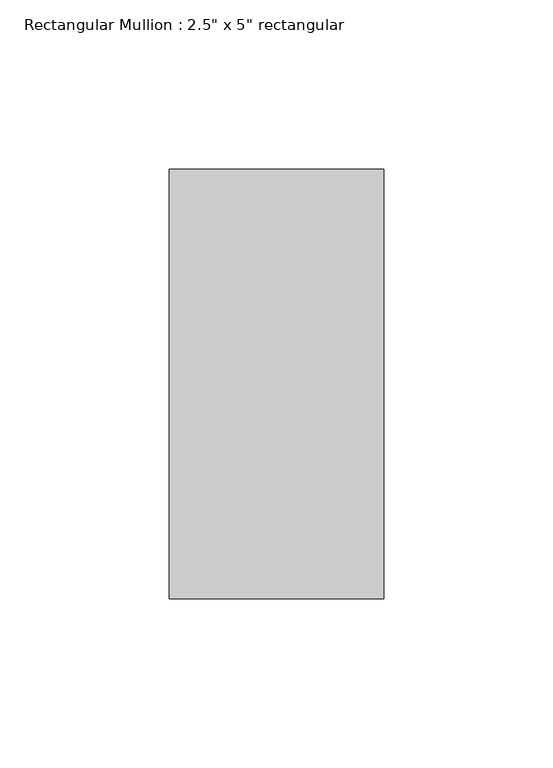
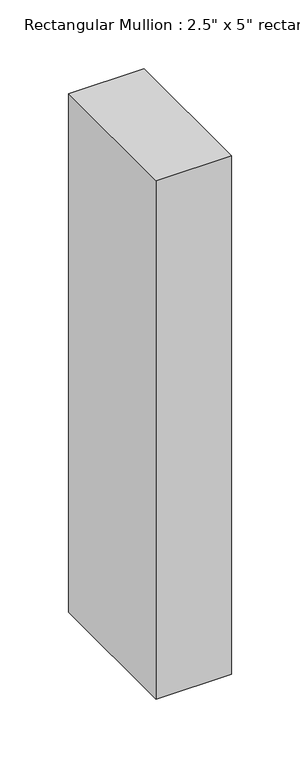
"""IFC4 building model written with IfcOpenShell, lengths in millimetres: member geometry."""

from ifc_helpers import new_model, si_unit, frame, origin, place, context, project, spatial, polyline, outline, extrude, source, transform, mapped, element, save


def member_40cdec31(model_context):
    return source(origin(), model_context, "Body", "SweptSolid", [
        extrude(outline(polyline([(0.0, 63.5), (0.0, -63.5), (-63.5, -63.5), (-63.5, 63.5), (0.0, 63.5)])), frame((0.0, 0.0, -460.375), z_axis=(0.0, 0.0, 1.0), x_axis=(1.0, 0.0, 0.0)), (0.0, 0.0, 1.0), 460.375),
    ])


if __name__ == "__main__":
    model = new_model("IFC4")
    model_context = context("Model", 3, world=origin())
    ifc_project = project(units=[si_unit("LENGTHUNIT", "METRE", prefix="MILLI")], contexts=[model_context])
    site = spatial("IfcSite", under=ifc_project)
    building = spatial("IfcBuilding", under=site)
    placement = place(None, origin())
    member_shape = member_40cdec31(model_context)
    element("IfcMember", 1, ObjectType="Rectangular Mullion : 2.5\" x 5\" rectangular", at=placement, inside=building, context=model_context, shape_type="MappedRepresentation", body=[
        mapped(member_shape, transform((0.0, 0.0, 0.0), x_axis=(1.0, 0.0, 0.0), y_axis=(0.0, 1.0, 0.0), z_axis=(0.0, 0.0, 1.0))),
    ])
    save(model, "model.ifc")

# Revit data of these elements
# Type "Rectangular Mullion : 2.5\" x 5\" rectangular"
#   built-in parameter 1007304 = 0.416667 (stored number, unit not read)
#   built-in parameter 1007301 = 0.104167 (stored number, unit not read)
#   built-in parameter 1007300 = 0.104167 (stored number, unit not read)
# Element 1 (IfcMember, "Rectangular Mullion : 2.5\" x 5\" rectangular")
#   Materials on its faces: "Aluminum"
# Materials
#   "Aluminum": class "Metal", colour RGB 247 247 247, transparency 0, Description = "Aluminum 6061", Cost = 0
